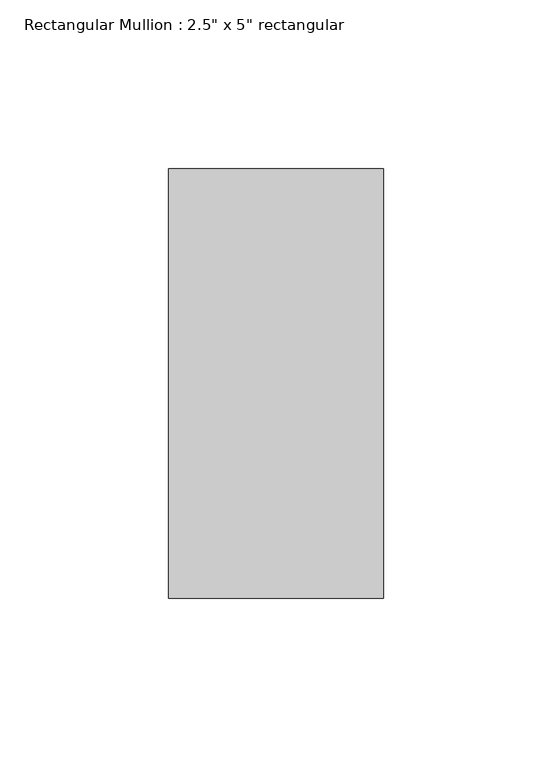
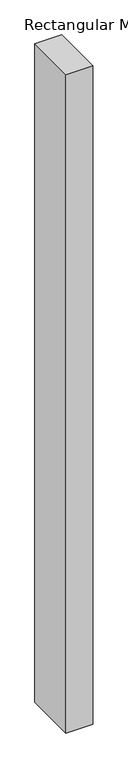
"""IFC4 building model written with IfcOpenShell, lengths in millimetres: member geometry."""

from ifc_helpers import new_model, si_unit, frame, origin, place, context, project, spatial, polyline, outline, extrude, source, transform, mapped, element, save


def member_194281bb(model_context):
    return source(origin(), model_context, "Body", "SweptSolid", [
        extrude(outline(polyline([(31.75, 63.5), (31.75, -63.5), (-31.75, -63.5), (-31.75, 63.5), (31.75, 63.5)])), frame((0.0, 0.0, -1644.7338557), z_axis=(0.0, 0.0, 1.0), x_axis=(1.0, 0.0, 0.0)), (0.0, 0.0, 1.0), 1644.7338557),
    ])


if __name__ == "__main__":
    model = new_model("IFC4")
    model_context = context("Model", 3, world=origin())
    ifc_project = project(units=[si_unit("LENGTHUNIT", "METRE", prefix="MILLI")], contexts=[model_context])
    site = spatial("IfcSite", under=ifc_project)
    building = spatial("IfcBuilding", under=site)
    placement = place(None, origin())
    member_shape = member_194281bb(model_context)
    element("IfcMember", 1, ObjectType="Rectangular Mullion : 2.5\" x 5\" rectangular", at=placement, inside=building, context=model_context, shape_type="MappedRepresentation", body=[
        mapped(member_shape, transform((0.0, 0.0, 0.0), x_axis=(1.0, 0.0, 0.0), y_axis=(0.0, 1.0, 0.0), z_axis=(0.0, 0.0, 1.0))),
    ])
    save(model, "model.ifc")

# Revit data of these elements
# Type "Rectangular Mullion : 2.5\" x 5\" rectangular"
#   built-in parameter 1007304 = 0.416667 (stored number, unit not read)
#   built-in parameter 1007301 = 0.104167 (stored number, unit not read)
#   built-in parameter 1007300 = 0.104167 (stored number, unit not read)
# Element 1 (IfcMember, "Rectangular Mullion : 2.5\" x 5\" rectangular")
#   Materials on its faces: "Aluminum"
# Materials
#   "Aluminum": class "Metal", colour RGB 247 247 247, transparency 0, Description = "Aluminum 6061", Cost = 0
